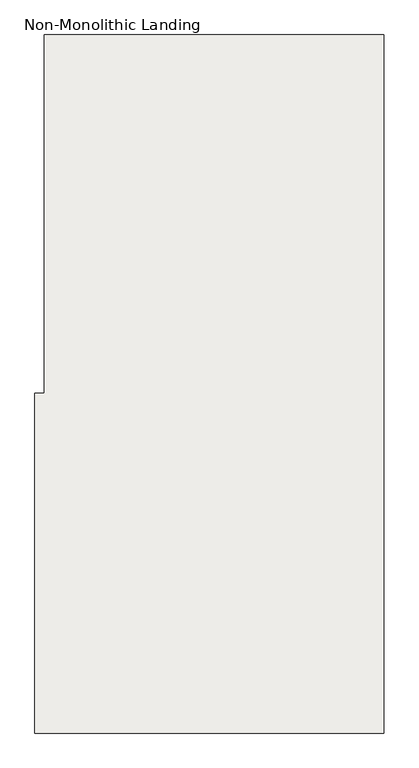
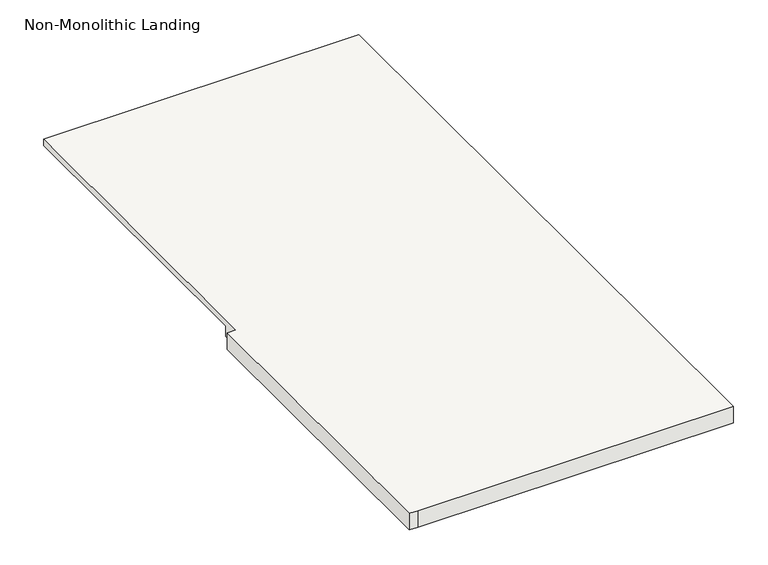
"""IFC4 building model written with IfcOpenShell, lengths in millimetres: slab geometry, Non-Monolithic Landing."""

from ifc_helpers import new_model, si_unit, origin, place, context, project, spatial, faceted_brep, source, transform, mapped, element, save


def non_monolithic_landing_284a18c3(model_context):
    return source(origin(), model_context, "Body", "Brep", [
        faceted_brep([(-1680.9866603, -2535.9331121, 1335.6166667), (-1655.5866603, -2535.9331121, 1310.2166667), (-1655.5866603, -3450.3331121, 1310.2166667), (-1680.9866603, -3450.3331121, 1335.6166667), (-1680.9866603, -3501.1331121, 1354.6666667), (-1706.3866603, -3501.1331121, 1354.6666667), (-1706.3866603, -4415.5331121, 1354.6666667), (-1680.9866603, -4415.5331121, 1354.6666667), (-766.5866603, -4415.5331121, 1354.6666667), (-766.5866603, -2535.9331121, 1354.6666667), (-1680.9866603, -2535.9331121, 1354.6666667), (-1655.5866603, -3450.3331121, 1303.8666667), (-1655.5866603, -2535.9331121, 1303.8666667), (-766.5866603, -2535.9331121, 1303.8666667), (-766.5866603, -4415.5331121, 1303.8666667), (-1680.9866603, -4415.5331121, 1303.8666667), (-1706.3866603, -4415.5331121, 1303.8666667), (-1706.3866603, -3501.1331121, 1303.8666667), (-1680.9866603, -3501.1331121, 1303.8666667), (-1680.9866603, -3450.3331121, 1303.8666667)], [[[0, 1, 2, 3]], [[4, 5, 6, 7, 8, 9, 10]], [[11, 12, 13, 14, 15, 16, 17, 18, 19]], [[12, 11, 2, 1]], [[11, 19, 3, 2]], [[4, 10, 0, 3, 19, 18]], [[5, 4, 18, 17]], [[6, 5, 17, 16]], [[7, 6, 16, 15]], [[8, 7, 15, 14]], [[9, 8, 14, 13]], [[10, 9, 13, 12, 1, 0]]]),
    ])


if __name__ == "__main__":
    model = new_model("IFC4")
    model_context = context("Model", 3, world=origin())
    ifc_project = project(units=[si_unit("LENGTHUNIT", "METRE", prefix="MILLI")], contexts=[model_context])
    site = spatial("IfcSite", under=ifc_project)
    building = spatial("IfcBuilding", under=site)
    placement = place(None, origin())
    non_monolithic_landing_shape = non_monolithic_landing_284a18c3(model_context)
    element("IfcSlab", 1, ObjectType="Non-Monolithic Landing", at=placement, inside=building, context=model_context, shape_type="MappedRepresentation", body=[
        mapped(non_monolithic_landing_shape, transform((0.0, 0.0, 0.0), x_axis=(1.0, 0.0, 0.0), y_axis=(0.0, 1.0, 0.0), z_axis=(0.0, 0.0, 1.0))),
    ])
    save(model, "model.ifc")
